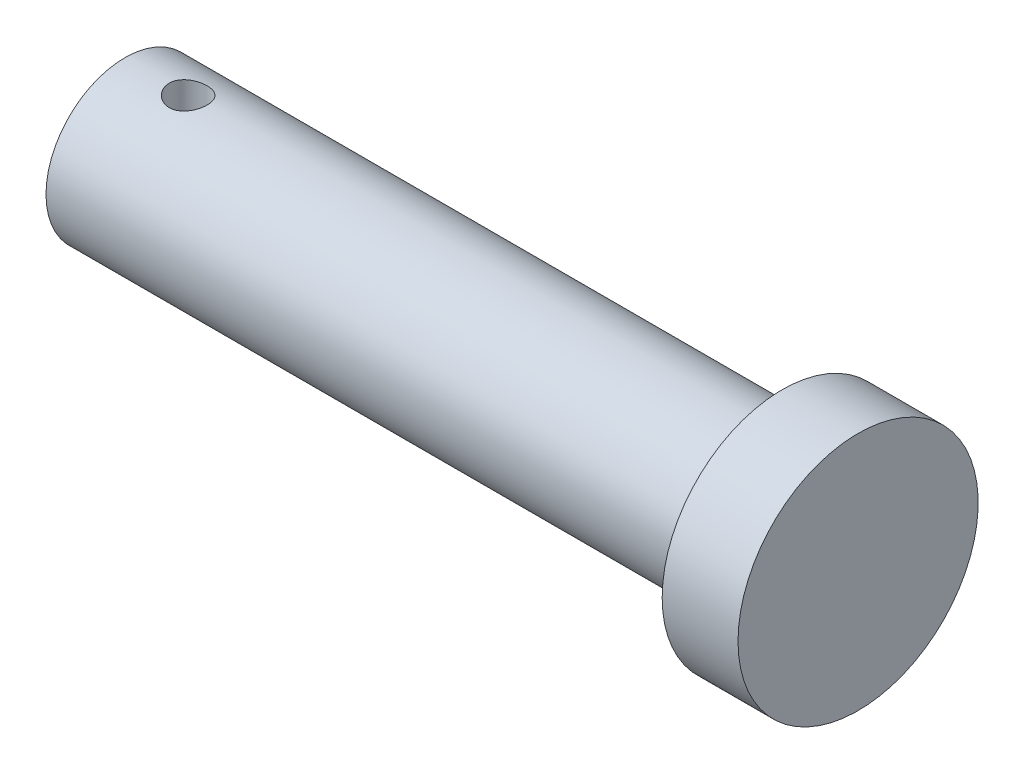
from build123d import *

# Parameters (mm, degrees)
CROSS_HOLE_6_DEPTH      = 120.071407147
CROSS_HOLE_6_DEPTH_BACK = 120.071407147
CROSS_HOLE_SKETCH_R     = 3


with BuildPart() as part:
    # Pin Profile Sketch → Headed Pin Body (revolve)
    with BuildSketch(Plane.XY, mode=Mode.PRIVATE) as headed_pin_body_sk:
        Polygon((0, 0), (84, 0), (116, 0), (116, -19), (104, -19), (104, -12.5), (0, -12.5), align=None)
    revolve(headed_pin_body_sk.sketch.rotate(Axis((-210, 0, 0), (1, 0, 0)), 270), axis=Axis((-210, 0, 0), (1, 0, 0)))

    # Cross Hole Sketch → Cross Hole Ø6 (cut, two sides: drawn at the far end of the back side and taken through both)
    with BuildSketch(Plane(origin=(0, 0, 0), x_dir=(1, 0, 0), z_dir=(0, 1, 0)).offset(-CROSS_HOLE_6_DEPTH_BACK)):
        with Locations(Location((10, 0, 0), (0, 0, 270))):
            Circle(CROSS_HOLE_SKETCH_R)
    extrude(amount=CROSS_HOLE_6_DEPTH + CROSS_HOLE_6_DEPTH_BACK, mode=Mode.SUBTRACT)


solid = part.part
